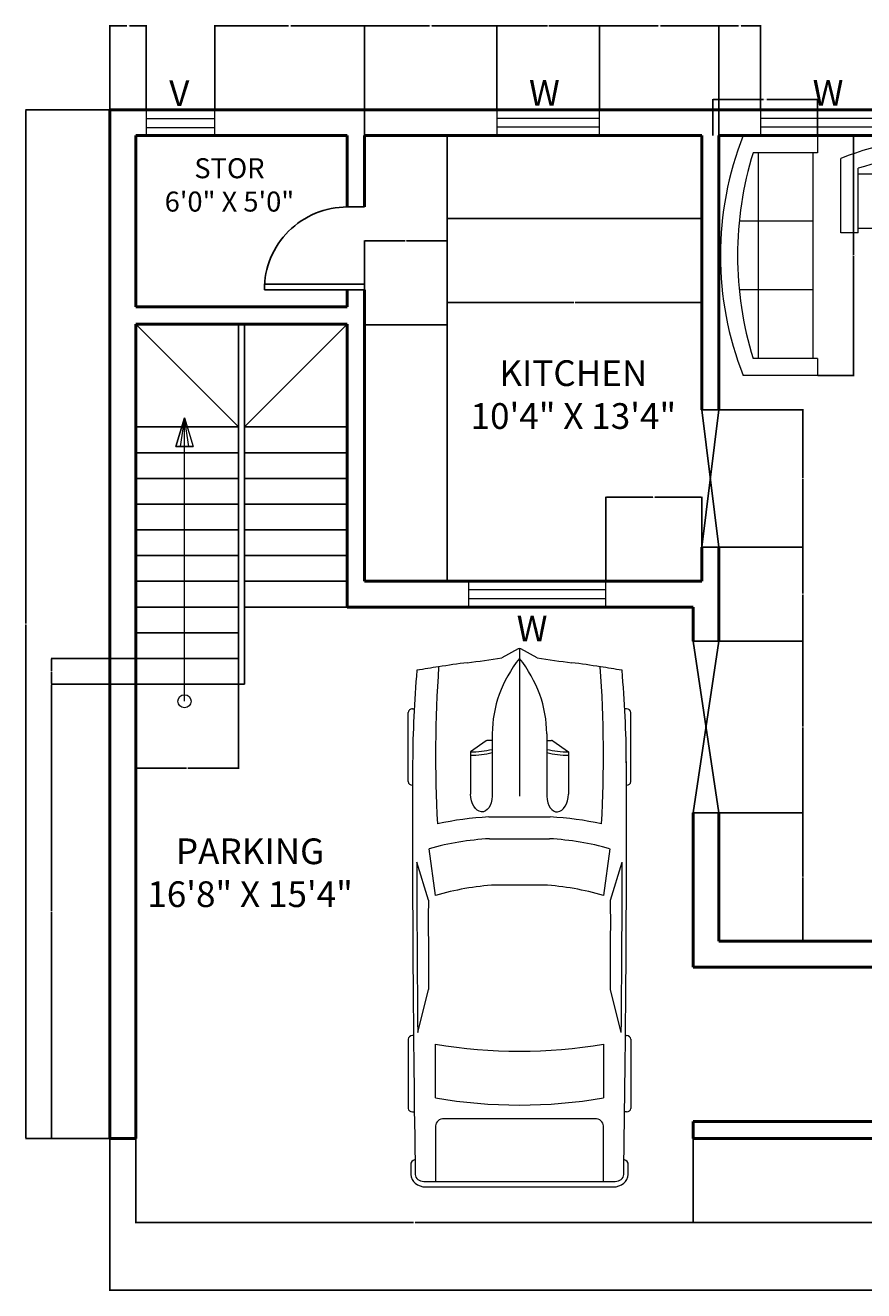
# Model space of a CAD drawing. Units: inches. Extents: x 1727 to 2326, y 1693 to 2164.
# Tile 1 of 3: x 1727 to 2020, y 1693 to 2136. Entities that reach past the tile are written whole.
import ezdxf

# ---------------------------------------------------------------- set-up
doc = ezdxf.new("R2010")
doc.units = ezdxf.units.IN
for name, color, linetype, lineweight in [('A-ANNO-DIMS', 2, 'Continuous', 18), ('A-ANNO-SYMB', 2, 'Continuous', 18), ('A-ANNO-TEXT', 3, 'Continuous', 18), ('A-AREA-IDEN', 7, 'Continuous', 25), ('A-DOOR', 3, 'Continuous', 25), ('A-EQPM-VEHI', 8, 'Continuous', 13), ('A-FLOR-CASE', 9, 'Continuous', 25), ('A-FLOR-STRS', 7, 'Continuous', 25), ('A-FURN', 8, 'Continuous', 18), ('A-GLAZ', 4, 'Continuous', 18), ('A-WALL', 7, 'Continuous', 50)]:
    doc.layers.add(name, color=color, linetype=linetype, lineweight=lineweight)
doc.styles.add('Annotative', font='arial.ttf')
doc.styles.get("Standard").update_dxf_attribs({"font": 'arial.ttf'})
doc.dimstyles.get("Standard").update_dxf_attribs({"dimtxt": 0.18, "dimasz": 0.18, "dimexe": 0.18, "dimexo": 0.0625, "dimgap": 0.09, "dimtad": 0, "dimtih": 1, "dimtoh": 1, "dimdec": 4, "dimzin": 0, "dimdsep": 46, "dimtxsty": 'Standard', "dimcen": 0.09, "dimadec": 0, "dimazin": 0, "dimtfac": 1, "dimtdec": 4, "dimtofl": 0, "dimtmove": 0, "dimatfit": 3, "dimfxl": 1, "dimtolj": 1, "dimtzin": 0, "dimarcsym": 0})

# ---------------------------------------------------------------- blocks, each defined once
blk = doc.blocks.new('Sofa - Roundback 7 ft.')
for p, q in [((-12.00002, -32.4421), (-12.00003, -6.5971)), ((11.99997, -32.4421), (11.99998, -6.5971)), ((-36.000027, -34), (-36.000027, -11.4696)), ((35.99998, -34), (35.99998, -11.4696)), ((-35.999844, -13.3819), (35.9998, -13.3819)), ((-36.000027, -32.4421), (35.99998, -32.4421))]:
    blk.add_line(p, q)
for points in [[(-36.000027, -34), (-42.000027, -34), (-42.000027, -8)], [(41.99998, -8), (41.99998, -34), (35.99998, -34)]]:
    blk.add_lwpolyline(points)
for centre, radius, start, end in [((0, -114.25), 114.25, 68.43141, 111.5686), ((-0.00001, -127.1968), 121.1968, 72.72033, 107.2797)]:
    blk.add_arc(centre, radius, start, end)
blk = doc.blocks.new('*U8')
for p, q in [((21.1, 37.41), (21.1, 36.83)), ((46.55, 38.89), (22.35, 38.89)), ((47.8, 37.39), (47.8, 37.41)), ((87.99, 31.87), (74.76, 35.92)), ((134.31, 35.6), (119.29, 31.78)), ((135.45, 37.07), (135.45, 37.41)), ((136.7, 38.89), (160.9, 38.89)), ((162.15, 37.41), (162.15, 36.77)), ((70.03, 31.54), (86.41, 29.35)), ((186.47, -33.5), (186.47, 33.5)), ((188.4, -32.76), (188.4, 32.76)), ((138.42, 29.35), (157.25, 29.35)), ((186.47, 29.35), (167.01, 29.35)), ((164.52, 26.39), (164.52, -26.39)), ((32.27, 11.63), (36.13, 17.17)), ((36.13, 17.17), (50.94, 17.17)), ((29.77, 9.51), (51.68, 9.51)), ((32.12, 9.51), (32.12, 11.15)), ((58.92, -10.77), (58.92, 10.77)), ((66.55, -10.53), (66.55, 10.53)), ((186.47, -10.53), (186.47, 10.53)), ((3.27, 6.13), (0.1, 0.41)), ((82.74, 8.5), (82.74, -8.5)), ((0, 0), (51.68, 0)), ((0.1, -0.41), (3.27, -6.13)), ((29.77, -9.51), (51.68, -9.51)), ((32.12, -9.51), (32.12, -11.15)), ((32.27, -11.63), (36.13, -17.17)), ((36.13, -17.17), (50.94, -17.17)), ((86.41, -29.35), (70.03, -31.54)), ((157.25, -29.35), (138.42, -29.35)), ((167.01, -29.35), (186.47, -29.35)), ((87.99, -31.87), (74.76, -35.92)), ((134.31, -35.6), (119.29, -31.78)), ((21.1, -37.41), (21.1, -36.83)), ((46.55, -38.89), (22.35, -38.89)), ((47.8, -37.39), (47.8, -37.41)), ((135.45, -37.07), (135.45, -37.41)), ((136.7, -38.89), (160.9, -38.89)), ((162.15, -37.41), (162.15, -36.77))]:
    blk.add_line(p, q)
for centre, major_axis, ratio, start_param, end_param in [((266.03, -27.52), (0, 313.31), 0.842304, 1.367076, 1.39176), ((41.19, -490.86), (0, 528.23), 0.842304, 0.00281, 0.075598), ((22.35, 37.41), (0, -1.48), 0.842304, 3.141593, 4.712389), ((64.48, -10555.62), (0, 10593.03), 0.842304, -0.013397, 0.002797), ((46.55, 37.41), (0, 1.48), 0.842304, -1.570796, 0), ((64.48, -10555.62), (0, -10591.55), 0.842304, 3.133765, 3.140441), ((136.7, 37.41), (0, -1.48), 0.842304, 3.141593, 4.712389), ((160.9, 37.41), (0, 1.48), 0.842304, -1.570796, 0), ((180.63, 35.84), (0, 2.22), 0.842304, -0.013017, 1.249894), ((64.48, -10556.36), (0, 10595.31), 0.842304, -0.013397, -0.013017), ((183.98, 33.5), (0, -2.96), 0.842304, 1.570796, 3.128196), ((183.98, 32.76), (0, -5.25), 0.842304, 1.570796, 3.128196), ((135.29, 5.39), (0, 81.77), 0.842304, 1.245306, 1.50788), ((95.79, -3666.35), (0, -3698.24), 0.842304, 3.134049, 3.144098), ((259.18, -27.52), (0, -305.3), 0.842304, 4.528606, 4.561838), ((37.47, -593.96), (0, -623.33), 0.842304, 3.096046, 3.200911), ((134.4, 5.39), (0, -89.78), 0.842304, 4.449482, 4.652344), ((149.6, 2.8), (0, -79.58), 0.842304, 4.372215, 4.640744), ((17.08, 0), (0, 147.02), 0.842304, 4.511394, 4.913384), ((35.91, 0), (0, 147.02), 0.842304, 4.511394, 4.913384), ((167.01, 26.39), (0, 2.96), 0.842304, 0, 1.570796), ((-204.49, 52.4), (0, -250.96), 0.842304, 1.385369, 1.434372), ((13.04, 17.01), (0, 27.42), 0.842304, 4.435146, 4.718221), ((14.2, 17.01), (0, 27.42), 0.842304, 4.435146, 4.718221), ((50.79, 13.34), (6.34, -0.36), 0.603834, -1.395552, 1.581315), ((29.77, -46.66), (0, 56.17), 0.842304, 0, 0.590319), ((32.75, 11.15), (0, 0.74), 0.842304, 0.879714, 1.570796), ((0.62, 0), (0, -0.74), 0.842304, 4.131459, 5.293319), ((29.77, 46.66), (0, 56.17), 0.842304, 2.551274, 3.141593), ((-204.49, -52.4), (0, 250.96), 0.842304, -1.434372, -1.385369), ((149.6, -2.8), (0, -79.58), 0.842304, -1.499151, -1.230623), ((32.75, -11.15), (0, -0.74), 0.842304, 4.712389, 5.403472), ((13.04, -17.01), (0, -27.42), 0.842304, 1.564964, 1.848039), ((14.2, -17.01), (0, -27.42), 0.842304, 1.564964, 1.848039), ((134.4, -5.39), (0, -89.78), 0.842304, -1.510751, -1.307889), ((135.29, -5.39), (0, -81.77), 0.842304, -1.50788, -1.245306), ((259.18, 27.52), (0, 305.3), 0.842304, 1.721348, 1.754579), ((167.01, -26.39), (0, -2.96), 0.842304, 4.712389, 6.283185), ((266.03, 27.52), (0, 313.31), 0.842304, 1.749832, 1.774517), ((37.47, 593.96), (0, -623.33), 0.842304, -0.059319, 0.045547), ((95.79, 3666.35), (0, -3698.24), 0.842304, -0.002505, 0.007544), ((183.98, -33.5), (0, 2.96), 0.842304, 3.15499, 4.712389), ((183.98, -32.76), (0, -5.25), 0.842304, 0.013397, 1.570796), ((41.19, 490.86), (0, -528.23), 0.842304, -0.075598, -0.00281), ((22.35, -37.41), (0, 1.48), 0.842304, 1.570796, 3.141593), ((64.48, 10555.62), (0, 10593.03), 0.842304, 3.138796, 3.15499), ((46.55, -37.41), (0, -1.48), 0.842304, 0, 1.570796), ((64.48, 10555.62), (0, -10591.55), 0.842304, 0.001152, 0.007828), ((136.7, -37.41), (0, -1.48), 0.842304, -1.570796, 0), ((160.9, -37.41), (0, 1.48), 0.842304, 3.141593, 4.712389), ((180.63, -35.84), (0, -2.22), 0.842304, -1.249894, 0.013017), ((64.48, 10556.36), (0, 10595.31), 0.842304, 3.15461, 3.15499)]:
    blk.add_ellipse(centre, major_axis=major_axis, ratio=ratio, start_param=start_param, end_param=end_param)
at = {"extrusion": (0, 0, -1)}
blk.add_ellipse((50.79, -13.34), major_axis=(6.34, 0.36), ratio=0.603834, start_param=-1.395552, end_param=1.581315, dxfattribs=at)
blk = doc.blocks.new('WIN-48IN')
for p, q in [((0, 48), (0, 0)), ((9, 48), (0, 48)), ((3, 48), (3, 0)), ((6, 0), (6, 48)), ((9, 0), (9, 48)), ((0, 0), (9, 0))]:
    blk.add_line(p, q)
blk = doc.blocks.new('DOOR-SWING-29IN')
for p, q in [((0, 29), (0, 35)), ((2, 29), (2, 35)), ((29, 35), (29, 29)), ((0, 29), (0, 0)), ((2, 29), (2, 0))]:
    blk.add_line(p, q)
blk.add_arc((0, 29), 29, 270, 0)
blk = doc.blocks.new('*D17')
at = {"layer": 'A-ANNO-DIMS', "color": 0, "lineweight": -2, "transparency": 16777216}
for p, q in [((2003.94, 2097.38), (2016.66, 2097.38)), ((2016.48, 2097.2), (2016.48, 2055.56)), ((2016.48, 2013.56), (2016.48, 2055.2)), ((2003.94, 2013.38), (2016.66, 2013.38))]:
    blk.add_line(p, q, dxfattribs=at)
at = {"layer": 'A-ANNO-DIMS', "color": 0, "transparency": 16777216}
for points in [[(2016.45, 2097.2), (2016.51, 2097.2), (2016.48, 2097.38)], [(2016.45, 2013.56), (2016.51, 2013.56), (2016.48, 2013.38)]]:
    blk.add_solid(points, dxfattribs=at)
at = {"layer": 'Defpoints', "color": 0, "transparency": 16777216}
for p in [(2003.88, 2097.38), (2016.48, 2097.38), (2003.88, 2013.38)]:
    blk.add_point(p, dxfattribs=at)
at = {"layer": 'A-ANNO-DIMS', "color": 0, "transparency": 16777216, "insert": (2016.48, 2055.38), "char_height": 0.18, "attachment_point": 5}
blk.add_mtext('\\A1;SOFA 84 TYP.', dxfattribs=at)
blk = doc.blocks.new('*D18')
at = {"layer": 'A-ANNO-DIMS', "color": 0, "lineweight": -2, "transparency": 16777216}
for p, q in [((1967.21, 2097.44), (1967.21, 2110.16)), ((1967.39, 2109.98), (1985.01, 2109.98)), ((2003.7, 2109.98), (1986.07, 2109.98)), ((2003.88, 2097.44), (2003.88, 2110.16))]:
    blk.add_line(p, q, dxfattribs=at)
at = {"layer": 'A-ANNO-DIMS', "color": 0, "transparency": 16777216}
for points in [[(1967.39, 2110.01), (1967.39, 2109.95), (1967.21, 2109.98)], [(2003.7, 2110.01), (2003.7, 2109.95), (2003.88, 2109.98)]]:
    blk.add_solid(points, dxfattribs=at)
at = {"layer": 'Defpoints', "color": 0, "transparency": 16777216}
for p in [(1967.21, 2109.98), (1967.21, 2097.38), (2003.88, 2097.38)]:
    blk.add_point(p, dxfattribs=at)
at = {"layer": 'A-ANNO-DIMS', "color": 0, "transparency": 16777216, "insert": (1985.54, 2109.98), "char_height": 0.18, "attachment_point": 5}
blk.add_mtext('\\A1;37 TYP.', dxfattribs=at)
blk = doc.blocks.new('*D33')
at = {"layer": 'A-ANNO-DIMS', "color": 0, "lineweight": -2, "transparency": 16777216}
for p, q in [((1756.37, 1746.32), (1756.37, 1693.11)), ((2296.37, 1746.32), (2296.37, 1693.11)), ((1756.55, 1693.29), (2026.08, 1693.29)), ((2296.19, 1693.29), (2026.66, 1693.29))]:
    blk.add_line(p, q, dxfattribs=at)
at = {"layer": 'A-ANNO-DIMS', "color": 0, "transparency": 16777216}
for points in [[(1756.55, 1693.32), (1756.55, 1693.26), (1756.37, 1693.29)], [(2296.19, 1693.32), (2296.19, 1693.26), (2296.37, 1693.29)]]:
    blk.add_solid(points, dxfattribs=at)
at = {"layer": 'Defpoints', "color": 0, "transparency": 16777216}
for p in [(1756.37, 1746.38), (2296.37, 1746.38), (2296.37, 1693.29)]:
    blk.add_point(p, dxfattribs=at)
at = {"layer": 'A-ANNO-DIMS', "color": 0, "transparency": 16777216, "insert": (2026.37, 1693.29), "char_height": 0.18, "attachment_point": 5}
blk.add_mtext('\\A1;540', dxfattribs=at)
blk = doc.blocks.new('*D34')
at = {"layer": 'A-ANNO-DIMS', "color": 0, "lineweight": -2, "transparency": 16777216}
for p, q in [((1756.31, 2106.38), (1726.79, 2106.38)), ((1726.97, 2106.2), (1726.97, 1926.56)), ((1726.97, 1746.56), (1726.97, 1926.2)), ((1756.31, 1746.38), (1726.79, 1746.38))]:
    blk.add_line(p, q, dxfattribs=at)
at = {"layer": 'A-ANNO-DIMS', "color": 0, "transparency": 16777216}
for points in [[(1726.94, 2106.2), (1727, 2106.2), (1726.97, 2106.38)], [(1726.94, 1746.56), (1727, 1746.56), (1726.97, 1746.38)]]:
    blk.add_solid(points, dxfattribs=at)
at = {"layer": 'Defpoints', "color": 0, "transparency": 16777216}
for p in [(1726.97, 2106.38), (1756.37, 2106.38), (1756.37, 1746.38)]:
    blk.add_point(p, dxfattribs=at)
at = {"layer": 'A-ANNO-DIMS', "color": 0, "transparency": 16777216, "insert": (1726.97, 1926.38), "char_height": 0.18, "attachment_point": 5}
blk.add_mtext('\\A1;360', dxfattribs=at)
blk = doc.blocks.new('*D35')
at = {"layer": 'A-ANNO-DIMS', "color": 0, "lineweight": -2, "transparency": 16777216}
for p, q in [((1756.37, 2106.44), (1756.37, 2135.96)), ((1756.55, 2135.78), (1762.26, 2135.78)), ((1768.88, 2135.78), (1763.17, 2135.78)), ((1769.06, 2106.25), (1769.06, 2135.96))]:
    blk.add_line(p, q, dxfattribs=at)
at = {"layer": 'A-ANNO-DIMS', "color": 0, "transparency": 16777216}
for points in [[(1756.55, 2135.81), (1756.55, 2135.75), (1756.37, 2135.78)], [(1768.88, 2135.81), (1768.88, 2135.75), (1769.06, 2135.78)]]:
    blk.add_solid(points, dxfattribs=at)
at = {"layer": 'Defpoints', "color": 0, "transparency": 16777216}
for p in [(1769.06, 2135.78), (1756.37, 2106.38), (1769.06, 2106.18)]:
    blk.add_point(p, dxfattribs=at)
at = {"layer": 'A-ANNO-DIMS', "color": 0, "transparency": 16777216, "insert": (1762.71, 2135.78), "char_height": 0.18, "attachment_point": 5}
blk.add_mtext('\\A1;12.683', dxfattribs=at)
blk = doc.blocks.new('*D36')
at = {"layer": 'A-ANNO-DIMS', "color": 0, "lineweight": -2, "transparency": 16777216}
for p, q in [((1793.06, 2106.25), (1793.06, 2135.96)), ((1793.24, 2135.78), (1818.82, 2135.78)), ((1845.19, 2135.78), (1819.61, 2135.78)), ((1845.37, 2097.44), (1845.37, 2135.96))]:
    blk.add_line(p, q, dxfattribs=at)
at = {"layer": 'A-ANNO-DIMS', "color": 0, "transparency": 16777216}
for points in [[(1793.24, 2135.81), (1793.24, 2135.75), (1793.06, 2135.78)], [(1845.19, 2135.81), (1845.19, 2135.75), (1845.37, 2135.78)]]:
    blk.add_solid(points, dxfattribs=at)
at = {"layer": 'Defpoints', "color": 0, "transparency": 16777216}
for p in [(1845.37, 2135.78), (1793.06, 2106.18), (1845.37, 2097.38)]:
    blk.add_point(p, dxfattribs=at)
at = {"layer": 'A-ANNO-DIMS', "color": 0, "transparency": 16777216, "insert": (1819.21, 2135.78), "char_height": 0.18, "attachment_point": 5}
blk.add_mtext('\\A1;52.32', dxfattribs=at)
blk = doc.blocks.new('*D37')
at = {"layer": 'A-ANNO-DIMS', "color": 0, "lineweight": -2, "transparency": 16777216}
for p, q in [((1845.37, 2097.44), (1845.37, 2135.96)), ((1845.55, 2135.78), (1868.11, 2135.78)), ((1891.45, 2135.78), (1868.9, 2135.78)), ((1891.63, 2106.44), (1891.63, 2135.96))]:
    blk.add_line(p, q, dxfattribs=at)
at = {"layer": 'A-ANNO-DIMS', "color": 0, "transparency": 16777216}
for points in [[(1845.55, 2135.81), (1845.55, 2135.75), (1845.37, 2135.78)], [(1891.45, 2135.81), (1891.45, 2135.75), (1891.63, 2135.78)]]:
    blk.add_solid(points, dxfattribs=at)
at = {"layer": 'Defpoints', "color": 0, "transparency": 16777216}
for p in [(1891.63, 2135.78), (1891.63, 2106.38), (1845.37, 2097.38)]:
    blk.add_point(p, dxfattribs=at)
at = {"layer": 'A-ANNO-DIMS', "color": 0, "transparency": 16777216, "insert": (1868.5, 2135.78), "char_height": 0.18, "attachment_point": 5}
blk.add_mtext('\\A1;46.26', dxfattribs=at)
blk = doc.blocks.new('*D38')
at = {"layer": 'A-ANNO-DIMS', "color": 0, "lineweight": -2, "transparency": 16777216}
for p, q in [((1891.63, 2106.44), (1891.63, 2135.96)), ((1891.81, 2135.78), (1909.42, 2135.78)), ((1927.45, 2135.78), (1909.85, 2135.78)), ((1927.63, 2106.44), (1927.63, 2135.96))]:
    blk.add_line(p, q, dxfattribs=at)
at = {"layer": 'A-ANNO-DIMS', "color": 0, "transparency": 16777216}
for points in [[(1891.81, 2135.81), (1891.81, 2135.75), (1891.63, 2135.78)], [(1927.45, 2135.81), (1927.45, 2135.75), (1927.63, 2135.78)]]:
    blk.add_solid(points, dxfattribs=at)
at = {"layer": 'Defpoints', "color": 0, "transparency": 16777216}
for p in [(1927.63, 2135.78), (1891.63, 2106.38), (1927.63, 2106.38)]:
    blk.add_point(p, dxfattribs=at)
at = {"layer": 'A-ANNO-DIMS', "color": 0, "transparency": 16777216, "insert": (1909.63, 2135.78), "char_height": 0.18, "attachment_point": 5}
blk.add_mtext('\\A1;36', dxfattribs=at)
blk = doc.blocks.new('*D39')
at = {"layer": 'A-ANNO-DIMS', "color": 0, "lineweight": -2, "transparency": 16777216}
for p, q in [((1927.63, 2106.44), (1927.63, 2135.96)), ((1927.81, 2135.78), (1948.11, 2135.78)), ((1969.19, 2135.78), (1948.9, 2135.78)), ((1969.37, 2097.44), (1969.37, 2135.96))]:
    blk.add_line(p, q, dxfattribs=at)
at = {"layer": 'A-ANNO-DIMS', "color": 0, "transparency": 16777216}
for points in [[(1927.81, 2135.81), (1927.81, 2135.75), (1927.63, 2135.78)], [(1969.19, 2135.81), (1969.19, 2135.75), (1969.37, 2135.78)]]:
    blk.add_solid(points, dxfattribs=at)
at = {"layer": 'Defpoints', "color": 0, "transparency": 16777216}
for p in [(1969.37, 2135.78), (1927.63, 2106.38), (1969.37, 2097.38)]:
    blk.add_point(p, dxfattribs=at)
at = {"layer": 'A-ANNO-DIMS', "color": 0, "transparency": 16777216, "insert": (1948.5, 2135.78), "char_height": 0.18, "attachment_point": 5}
blk.add_mtext('\\A1;41.74', dxfattribs=at)
blk = doc.blocks.new('*D40')
at = {"layer": 'A-ANNO-DIMS', "color": 0, "lineweight": -2, "transparency": 16777216}
for p, q in [((1969.37, 2097.44), (1969.37, 2135.96)), ((1969.55, 2135.78), (1976.2, 2135.78)), ((1983.76, 2135.78), (1977.11, 2135.78)), ((1983.94, 2106.44), (1983.94, 2135.96))]:
    blk.add_line(p, q, dxfattribs=at)
at = {"layer": 'A-ANNO-DIMS', "color": 0, "transparency": 16777216}
for points in [[(1969.55, 2135.81), (1969.55, 2135.75), (1969.37, 2135.78)], [(1983.76, 2135.81), (1983.76, 2135.75), (1983.94, 2135.78)]]:
    blk.add_solid(points, dxfattribs=at)
at = {"layer": 'Defpoints', "color": 0, "transparency": 16777216}
for p in [(1983.94, 2135.78), (1983.94, 2106.38), (1969.37, 2097.38)]:
    blk.add_point(p, dxfattribs=at)
at = {"layer": 'A-ANNO-DIMS', "color": 0, "transparency": 16777216, "insert": (1976.65, 2135.78), "char_height": 0.18, "attachment_point": 5}
blk.add_mtext('\\A1;14.563', dxfattribs=at)
blk = doc.blocks.new('*D51')
at = {"layer": 'A-ANNO-DIMS', "color": 0, "lineweight": -2, "transparency": 16777216}
for p, q in [((1765.37, 1905.32), (1765.37, 1875.8)), ((1801.37, 1905.32), (1801.37, 1875.8)), ((1765.55, 1875.98), (1783.15, 1875.98)), ((1801.19, 1875.98), (1783.59, 1875.98))]:
    blk.add_line(p, q, dxfattribs=at)
at = {"layer": 'A-ANNO-DIMS', "color": 0, "transparency": 16777216}
for points in [[(1765.55, 1876.01), (1765.55, 1875.95), (1765.37, 1875.98)], [(1801.19, 1876.01), (1801.19, 1875.95), (1801.37, 1875.98)]]:
    blk.add_solid(points, dxfattribs=at)
at = {"layer": 'Defpoints', "color": 0, "transparency": 16777216}
for p in [(1765.37, 1905.38), (1801.37, 1905.38), (1765.37, 1875.98)]:
    blk.add_point(p, dxfattribs=at)
at = {"layer": 'A-ANNO-DIMS', "color": 0, "transparency": 16777216, "insert": (1783.37, 1875.98), "char_height": 0.18, "attachment_point": 5}
blk.add_mtext('\\A1;36', dxfattribs=at)
blk = doc.blocks.new('*D52')
at = {"layer": 'A-ANNO-DIMS', "color": 0, "lineweight": -2, "transparency": 16777216}
for p, q in [((1765.31, 1914.38), (1735.79, 1914.38)), ((1735.97, 1914.2), (1735.97, 1910.06)), ((1735.97, 1905.56), (1735.97, 1909.7)), ((1765.31, 1905.38), (1735.79, 1905.38))]:
    blk.add_line(p, q, dxfattribs=at)
at = {"layer": 'A-ANNO-DIMS', "color": 0, "transparency": 16777216}
for points in [[(1735.94, 1914.2), (1736, 1914.2), (1735.97, 1914.38)], [(1735.94, 1905.56), (1736, 1905.56), (1735.97, 1905.38)]]:
    blk.add_solid(points, dxfattribs=at)
at = {"layer": 'Defpoints', "color": 0, "transparency": 16777216}
for p in [(1735.97, 1914.38), (1765.37, 1914.38), (1765.37, 1905.38)]:
    blk.add_point(p, dxfattribs=at)
at = {"layer": 'A-ANNO-DIMS', "color": 0, "transparency": 16777216, "insert": (1735.97, 1909.88), "char_height": 0.18, "attachment_point": 5}
blk.add_mtext('\\A1;9', dxfattribs=at)
blk = doc.blocks.new('*D53')
at = {"layer": 'A-ANNO-DIMS', "color": 0, "lineweight": -2, "transparency": 16777216}
for p, q in [((1765.31, 1905.38), (1735.79, 1905.38)), ((1735.97, 1905.2), (1735.97, 1826.06)), ((1735.97, 1746.56), (1735.97, 1825.7)), ((1765.31, 1746.38), (1735.79, 1746.38))]:
    blk.add_line(p, q, dxfattribs=at)
at = {"layer": 'A-ANNO-DIMS', "color": 0, "transparency": 16777216}
for points in [[(1735.94, 1905.2), (1736, 1905.2), (1735.97, 1905.38)], [(1735.94, 1746.56), (1736, 1746.56), (1735.97, 1746.38)]]:
    blk.add_solid(points, dxfattribs=at)
at = {"layer": 'Defpoints', "color": 0, "transparency": 16777216}
for p in [(1735.97, 1905.38), (1765.37, 1905.38), (1765.37, 1746.38)]:
    blk.add_point(p, dxfattribs=at)
at = {"layer": 'A-ANNO-DIMS', "color": 0, "transparency": 16777216, "insert": (1735.97, 1825.88), "char_height": 0.18, "attachment_point": 5}
blk.add_mtext('\\A1;159', dxfattribs=at)
blk = doc.blocks.new('*D55')
at = {"layer": 'A-ANNO-DIMS', "color": 0, "lineweight": -2, "transparency": 16777216}
for p, q in [((1765.37, 1746.32), (1765.37, 1716.8)), ((1960.37, 1746.32), (1960.37, 1716.8)), ((1765.55, 1716.98), (1862.59, 1716.98)), ((1960.19, 1716.98), (1863.15, 1716.98))]:
    blk.add_line(p, q, dxfattribs=at)
at = {"layer": 'A-ANNO-DIMS', "color": 0, "transparency": 16777216}
for points in [[(1765.55, 1717.01), (1765.55, 1716.95), (1765.37, 1716.98)], [(1960.19, 1717.01), (1960.19, 1716.95), (1960.37, 1716.98)]]:
    blk.add_solid(points, dxfattribs=at)
at = {"layer": 'Defpoints', "color": 0, "transparency": 16777216}
for p in [(1765.37, 1746.38), (1960.37, 1746.38), (1765.37, 1716.98)]:
    blk.add_point(p, dxfattribs=at)
at = {"layer": 'A-ANNO-DIMS', "color": 0, "transparency": 16777216, "insert": (1862.87, 1716.98), "char_height": 0.18, "attachment_point": 5}
blk.add_mtext('\\A1;195', dxfattribs=at)
blk = doc.blocks.new('*D56')
at = {"layer": 'A-ANNO-DIMS', "color": 0, "lineweight": -2, "transparency": 16777216}
for p, q in [((1960.37, 1746.32), (1960.37, 1716.8)), ((2134.37, 1746.32), (2134.37, 1716.8)), ((1960.55, 1716.98), (2047.09, 1716.98)), ((2134.19, 1716.98), (2047.65, 1716.98))]:
    blk.add_line(p, q, dxfattribs=at)
at = {"layer": 'A-ANNO-DIMS', "color": 0, "transparency": 16777216}
for points in [[(1960.55, 1717.01), (1960.55, 1716.95), (1960.37, 1716.98)], [(2134.19, 1717.01), (2134.19, 1716.95), (2134.37, 1716.98)]]:
    blk.add_solid(points, dxfattribs=at)
at = {"layer": 'Defpoints', "color": 0, "transparency": 16777216}
for p in [(1960.37, 1746.38), (2134.37, 1746.38), (1960.37, 1716.98)]:
    blk.add_point(p, dxfattribs=at)
at = {"layer": 'A-ANNO-DIMS', "color": 0, "transparency": 16777216, "insert": (2047.37, 1716.98), "char_height": 0.18, "attachment_point": 5}
blk.add_mtext('\\A1;174', dxfattribs=at)
blk = doc.blocks.new('*D59')
at = {"layer": 'A-ANNO-DIMS', "color": 0, "lineweight": -2, "transparency": 16777216}
for p, q in [((1969.44, 2001.38), (1998.95, 2001.38)), ((1998.77, 2001.2), (1998.77, 1977.56)), ((1998.77, 1953.56), (1998.77, 1977.2)), ((1969.44, 1953.38), (1998.95, 1953.38))]:
    blk.add_line(p, q, dxfattribs=at)
at = {"layer": 'A-ANNO-DIMS', "color": 0, "transparency": 16777216}
for points in [[(1998.74, 2001.2), (1998.8, 2001.2), (1998.77, 2001.38)], [(1998.74, 1953.56), (1998.8, 1953.56), (1998.77, 1953.38)]]:
    blk.add_solid(points, dxfattribs=at)
at = {"layer": 'Defpoints', "color": 0, "transparency": 16777216}
for p in [(1969.37, 2001.38), (1969.37, 1953.38), (1998.77, 1953.38)]:
    blk.add_point(p, dxfattribs=at)
at = {"layer": 'A-ANNO-DIMS', "color": 0, "transparency": 16777216, "insert": (1998.77, 1977.38), "char_height": 0.18, "attachment_point": 5}
blk.add_mtext('\\A1;48', dxfattribs=at)
blk = doc.blocks.new('*D60')
at = {"layer": 'A-ANNO-DIMS', "color": 0, "lineweight": -2, "transparency": 16777216}
for p, q in [((1969.44, 1953.38), (1998.95, 1953.38)), ((1998.77, 1953.2), (1998.77, 1937.06)), ((1998.77, 1920.56), (1998.77, 1936.7)), ((1969.44, 1920.38), (1998.95, 1920.38))]:
    blk.add_line(p, q, dxfattribs=at)
at = {"layer": 'A-ANNO-DIMS', "color": 0, "transparency": 16777216}
for points in [[(1998.74, 1953.2), (1998.8, 1953.2), (1998.77, 1953.38)], [(1998.74, 1920.56), (1998.8, 1920.56), (1998.77, 1920.38)]]:
    blk.add_solid(points, dxfattribs=at)
at = {"layer": 'Defpoints', "color": 0, "transparency": 16777216}
for p in [(1969.37, 1953.38), (1969.37, 1920.38), (1998.77, 1920.38)]:
    blk.add_point(p, dxfattribs=at)
at = {"layer": 'A-ANNO-DIMS', "color": 0, "transparency": 16777216, "insert": (1998.77, 1936.88), "char_height": 0.18, "attachment_point": 5}
blk.add_mtext('\\A1;33', dxfattribs=at)
blk = doc.blocks.new('*D61')
at = {"layer": 'A-ANNO-DIMS', "color": 0, "lineweight": -2, "transparency": 16777216}
for p, q in [((1969.44, 1920.38), (1998.95, 1920.38)), ((1998.77, 1920.2), (1998.77, 1890.56)), ((1998.77, 1860.56), (1998.77, 1890.2)), ((1969.44, 1860.38), (1998.95, 1860.38))]:
    blk.add_line(p, q, dxfattribs=at)
at = {"layer": 'A-ANNO-DIMS', "color": 0, "transparency": 16777216}
for points in [[(1998.74, 1920.2), (1998.8, 1920.2), (1998.77, 1920.38)], [(1998.74, 1860.56), (1998.8, 1860.56), (1998.77, 1860.38)]]:
    blk.add_solid(points, dxfattribs=at)
at = {"layer": 'Defpoints', "color": 0, "transparency": 16777216}
for p in [(1969.37, 1920.38), (1969.37, 1860.38), (1998.77, 1860.38)]:
    blk.add_point(p, dxfattribs=at)
at = {"layer": 'A-ANNO-DIMS', "color": 0, "transparency": 16777216, "insert": (1998.77, 1890.38), "char_height": 0.18, "attachment_point": 5}
blk.add_mtext('\\A1;60', dxfattribs=at)
blk = doc.blocks.new('*D62')
at = {"layer": 'A-ANNO-DIMS', "color": 0, "lineweight": -2, "transparency": 16777216}
for p, q in [((1969.44, 1860.38), (1998.95, 1860.38)), ((1998.77, 1860.2), (1998.77, 1838.06)), ((1998.77, 1815.56), (1998.77, 1837.7)), ((1969.44, 1815.38), (1998.95, 1815.38))]:
    blk.add_line(p, q, dxfattribs=at)
at = {"layer": 'A-ANNO-DIMS', "color": 0, "transparency": 16777216}
for points in [[(1998.74, 1860.2), (1998.8, 1860.2), (1998.77, 1860.38)], [(1998.74, 1815.56), (1998.8, 1815.56), (1998.77, 1815.38)]]:
    blk.add_solid(points, dxfattribs=at)
at = {"layer": 'Defpoints', "color": 0, "transparency": 16777216}
for p in [(1969.37, 1860.38), (1969.37, 1815.38), (1998.77, 1815.38)]:
    blk.add_point(p, dxfattribs=at)
at = {"layer": 'A-ANNO-DIMS', "color": 0, "transparency": 16777216, "insert": (1998.77, 1837.88), "char_height": 0.18, "attachment_point": 5}
blk.add_mtext('\\A1;45', dxfattribs=at)
blk = doc.blocks.new('*D64')
at = {"layer": 'A-ANNO-DIMS', "color": 0, "lineweight": -2, "transparency": 16777216}
for p, q in [((1929.81, 1941.44), (1929.81, 1970.96)), ((1929.99, 1970.78), (1946.2, 1970.78)), ((1963.19, 1970.78), (1946.99, 1970.78)), ((1963.37, 1941.44), (1963.37, 1970.96))]:
    blk.add_line(p, q, dxfattribs=at)
at = {"layer": 'A-ANNO-DIMS', "color": 0, "transparency": 16777216}
for points in [[(1929.99, 1970.81), (1929.99, 1970.75), (1929.81, 1970.78)], [(1963.19, 1970.81), (1963.19, 1970.75), (1963.37, 1970.78)]]:
    blk.add_solid(points, dxfattribs=at)
at = {"layer": 'Defpoints', "color": 0, "transparency": 16777216}
for p in [(1963.37, 1970.78), (1929.81, 1941.38), (1963.37, 1941.38)]:
    blk.add_point(p, dxfattribs=at)
at = {"layer": 'A-ANNO-DIMS', "color": 0, "transparency": 16777216, "insert": (1946.59, 1970.78), "char_height": 0.18, "attachment_point": 5}
blk.add_mtext('\\A1;33.56', dxfattribs=at)
blk = doc.blocks.new('*D65')
at = {"layer": 'A-ANNO-DIMS', "color": 0, "lineweight": -2, "transparency": 16777216}
for p, q in [((1874.37, 2068.32), (1874.37, 2038.8)), ((1963.37, 2068.32), (1963.37, 2038.8)), ((1874.55, 2038.98), (1918.65, 2038.98)), ((1963.19, 2038.98), (1919.09, 2038.98))]:
    blk.add_line(p, q, dxfattribs=at)
at = {"layer": 'A-ANNO-DIMS', "color": 0, "transparency": 16777216}
for points in [[(1874.55, 2039.01), (1874.55, 2038.95), (1874.37, 2038.98)], [(1963.19, 2039.01), (1963.19, 2038.95), (1963.37, 2038.98)]]:
    blk.add_solid(points, dxfattribs=at)
at = {"layer": 'Defpoints', "color": 0, "transparency": 16777216}
for p in [(1874.37, 2068.38), (1963.37, 2068.38), (1874.37, 2038.98)]:
    blk.add_point(p, dxfattribs=at)
at = {"layer": 'A-ANNO-DIMS', "color": 0, "transparency": 16777216, "insert": (1918.87, 2038.98), "char_height": 0.18, "attachment_point": 5}
blk.add_mtext('\\A1;89', dxfattribs=at)
blk = doc.blocks.new('*D66')
at = {"layer": 'A-ANNO-DIMS', "color": 0, "lineweight": -2, "transparency": 16777216}
for p, q in [((1845.37, 2031.16), (1845.37, 2060.68)), ((1845.55, 2060.5), (1859.65, 2060.5)), ((1874.19, 2060.5), (1860.09, 2060.5)), ((1874.37, 2031.16), (1874.37, 2060.68))]:
    blk.add_line(p, q, dxfattribs=at)
at = {"layer": 'A-ANNO-DIMS', "color": 0, "transparency": 16777216}
for points in [[(1845.55, 2060.53), (1845.55, 2060.47), (1845.37, 2060.5)], [(1874.19, 2060.53), (1874.19, 2060.47), (1874.37, 2060.5)]]:
    blk.add_solid(points, dxfattribs=at)
at = {"layer": 'Defpoints', "color": 0, "transparency": 16777216}
for p in [(1874.37, 2060.5), (1845.37, 2031.1), (1874.37, 2031.1)]:
    blk.add_point(p, dxfattribs=at)
at = {"layer": 'A-ANNO-DIMS', "color": 0, "transparency": 16777216, "insert": (1859.87, 2060.5), "char_height": 0.18, "attachment_point": 5}
blk.add_mtext('\\A1;29', dxfattribs=at)

msp = doc.modelspace()

# ---------------------------------------------------------------- linework, layer by layer
at = {"layer": 'A-ANNO-SYMB'}
for p, q in [((1782.4415, 1998.5763), (1779.4415, 1988.5763)), ((1779.4415, 1988.5763), (1782.4415, 1998.5763)), ((1782.4415, 1998.5763), (1780.9415, 1988.5763)), ((1782.4415, 1988.5763), (1782.4415, 1998.5763)), ((1782.4415, 1998.5763), (1785.4415, 1988.5763)), ((1783.9415, 1988.5763), (1782.4415, 1998.5763)), ((1782.4415, 1988.5763), (1779.4415, 1988.5763)), ((1779.4415, 1988.5763), (1782.4415, 1988.5763)), ((1782.4415, 1899.3942), (1782.4415, 1988.5763)), ((1782.4415, 1988.5763), (1785.4415, 1988.5763)), ((1785.4415, 1988.5763), (1782.4415, 1988.5763)), ((1785.4415, 1988.5763), (1783.9415, 1988.5763))]:
    msp.add_line(p, q, dxfattribs=at)
msp.add_circle((1782.4415, 1899.3942), 2.2869, dxfattribs=at)
at = {"layer": 'A-DOOR'}
for p, q in [((1969.3729, 2001.3813), (1963.3729, 2001.3813)), ((1963.3729, 1953.3813), (1969.3729, 2001.3813)), ((1969.3729, 2001.3813), (1963.3729, 2001.3813)), ((1963.3729, 2001.3813), (1969.3729, 1953.3813)), ((1963.3729, 1953.3813), (1969.3729, 1953.3813)), ((1960.3729, 1920.3813), (1969.3729, 1920.3813)), ((1960.3729, 1860.3813), (1969.3729, 1920.3813)), ((1969.3729, 1920.3813), (1960.3729, 1920.3813)), ((1960.3729, 1920.3813), (1969.3729, 1860.3813)), ((1969.3729, 1860.3813), (1960.3729, 1860.3813))]:
    msp.add_line(p, q, dxfattribs=at)
at = {"layer": 'A-FLOR-CASE'}
for p, q in [((1874.3729, 2097.3813), (1874.3729, 2068.3813)), ((1874.3729, 2068.3813), (1963.3729, 2068.3813)), ((1845.3729, 2031.101), (1874.3729, 2031.101)), ((1874.3729, 2031.101), (1874.3729, 1941.3813))]:
    msp.add_line(p, q, dxfattribs=at)
at = {"layer": 'A-FLOR-STRS'}
for p, q in [((1801.3729, 1995.3813), (1765.3729, 2031.3813)), ((1765.3729, 2031.3813), (1786.3741, 2031.3813)), ((1801.3729, 1905.3813), (1801.3729, 2031.3813)), ((1803.3729, 1905.3813), (1803.3729, 2031.3813)), ((1803.3729, 1995.3813), (1839.3729, 2031.3813)), ((1765.3729, 1995.3813), (1801.3729, 1995.3813)), ((1803.3729, 1995.3813), (1839.3729, 1995.3813)), ((1765.3729, 1986.3813), (1801.3729, 1986.3813)), ((1803.3729, 1986.3813), (1839.3729, 1986.3813)), ((1765.3729, 1977.3813), (1801.3729, 1977.3813)), ((1803.3729, 1977.3813), (1839.3729, 1977.3813)), ((1765.3729, 1968.3813), (1801.3729, 1968.3813)), ((1803.3729, 1968.3813), (1839.3729, 1968.3813)), ((1765.3729, 1959.3813), (1801.3729, 1959.3813)), ((1803.3729, 1959.3813), (1839.3729, 1959.3813)), ((1765.3729, 1950.3813), (1801.3729, 1950.3813)), ((1803.3729, 1950.3813), (1839.3729, 1950.3813)), ((1765.3729, 1941.3813), (1801.3729, 1941.3813)), ((1803.3729, 1941.3813), (1839.3729, 1941.3813)), ((1765.3729, 1932.3813), (1801.3729, 1932.3813)), ((1803.3729, 1932.3813), (1839.3729, 1932.3813)), ((1765.3729, 1923.3813), (1801.3729, 1923.3813)), ((1765.3729, 1914.3813), (1801.3729, 1914.3813)), ((1765.3729, 1905.3813), (1803.3729, 1905.3813))]:
    msp.add_line(p, q, dxfattribs=at)
at = {"layer": 'A-GLAZ'}
for p, q in [((1769.0559, 2106.1833), (1769.0559, 2097.1833)), ((1793.0559, 2097.1833), (1793.0559, 2106.1833)), ((1927.6343, 2106.3813), (1879.6343, 2106.3813)), ((1891.6343, 2106.3813), (1891.6343, 2097.3813)), ((1927.6343, 2097.3813), (1927.6343, 2106.3813)), ((1793.0559, 2103.1833), (1769.0559, 2103.1833)), ((1769.0559, 2100.1833), (1793.0559, 2100.1833)), ((1927.6343, 2103.3813), (1891.6343, 2103.3813)), ((1891.6343, 2100.3813), (1927.6343, 2100.3813)), ((1879.6343, 2097.3813), (1927.6343, 2097.3813))]:
    msp.add_line(p, q, dxfattribs=at)
at = {"layer": 'A-WALL'}
for p, q in [((1756.3729, 2106.3813), (2296.3729, 2106.3813)), ((1756.3729, 1746.3813), (1756.3729, 2106.3813)), ((1756.3729, 2106.3813), (1765.3729, 2106.3813)), ((1765.3729, 2097.3813), (1839.3729, 2097.3813)), ((1765.3729, 2037.3813), (1765.3729, 2097.3813)), ((1839.3729, 2097.3813), (1839.3729, 2072.3813)), ((1845.3729, 2097.3813), (1845.3729, 2072.3813)), ((1845.3729, 2097.3813), (1963.3729, 2097.3813)), ((1963.3729, 2097.3813), (1963.3729, 2001.3813)), ((1969.3729, 2097.3813), (1969.3729, 2001.3813)), ((1969.3729, 2097.3813), (2137.3729, 2097.3813)), ((1839.3729, 2037.3813), (1839.3729, 2043.3813)), ((1839.3729, 2043.3813), (1839.3729, 2037.3813)), ((1845.3729, 2043.3813), (1845.3729, 1941.3813)), ((1765.3729, 2037.3813), (1839.3729, 2037.3813)), ((1765.3729, 1755.3813), (1765.3729, 2031.3813)), ((1765.3729, 2031.3813), (1839.3729, 2031.3813)), ((1839.3729, 2031.3813), (1839.3729, 1941.3813)), ((1963.3729, 1941.3813), (1963.3729, 1953.3813)), ((1963.3729, 1953.3813), (1963.3729, 1941.3813)), ((1969.3729, 1953.3813), (1969.3729, 1941.3813)), ((1839.3729, 1941.3813), (1839.3729, 1932.3813)), ((1845.3729, 1941.3813), (1963.3729, 1941.3813)), ((1969.3729, 1941.3813), (1969.3729, 1927.4801)), ((1839.3729, 1932.3813), (1960.3729, 1932.3813)), ((1960.3729, 1932.3813), (1960.3729, 1920.3813)), ((1960.3729, 1932.3813), (1960.3729, 1920.3813)), ((1969.3729, 1932.3813), (1969.3729, 1920.3813)), ((1960.3729, 1860.3813), (1960.3729, 1806.3813)), ((1969.3729, 1860.3813), (1969.3729, 1815.3813)), ((1969.3729, 1815.3813), (2047.3729, 1815.3813)), ((1963.3729, 1806.3813), (1960.3729, 1806.3813)), ((1963.3729, 1806.3813), (2134.3729, 1806.3813)), ((1765.3729, 1755.3813), (1765.3729, 1746.3813)), ((1960.3729, 1752.3813), (1960.3729, 1746.3813)), ((2134.3729, 1752.3813), (1960.3729, 1752.3813)), ((1765.3729, 1746.3813), (1756.3729, 1746.3813)), ((2296.3729, 1746.3813), (1960.3729, 1746.3813))]:
    msp.add_line(p, q, dxfattribs=at)

# ---------------------------------------------------------------- block references
at = {"layer": 'A-DOOR', "extrusion": (0, 0, -1), "zscale": -1, "rotation": 89.99999999999937}
msp.add_blockref('DOOR-SWING-29IN', (-1810.3726, 2043.3814), dxfattribs=at)
at = {"layer": 'A-EQPM-VEHI', "rotation": 270}
msp.add_blockref('*U8', (1899.6143, 1917.8239), dxfattribs=at)
at = {"layer": 'A-FURN'}
msp.add_blockref('Sofa - Roundback 7 ft.', (2054.0432, 2097.3813), dxfattribs=at)
at = {"layer": 'A-FURN', "rotation": 90}
msp.add_blockref('Sofa - Roundback 7 ft.', (1969.8756, 2055.3814), dxfattribs=at)
at = {"layer": 'A-GLAZ'}
for p, rotation in [((1983.936, 2106.3812), 270.0000000000012), ((1881.8142, 1941.3812), 269.9999999999983)]:
    msp.add_blockref('WIN-48IN', p, dxfattribs=dict(at, rotation=rotation))

# ---------------------------------------------------------------- texts
at = {"layer": 'A-ANNO-TEXT', "char_height": 9, "width": 33.967268, "attachment_point": 1, "style": 'Annotative'}
for s, insert in [('\\pxqc;V', (1763.6348, 2116.7193)), ('\\pxqc;W', (1891.3398, 2116.795)), ('\\pxqc;W', (1990.5516, 2116.8101)), ('\\pxqc;W', (1887.0324, 1929.3298))]:
    msp.add_mtext(s, dxfattribs=dict(at, insert=insert))
at = {"layer": 'A-AREA-IDEN', "attachment_point": 1, "style": 'Annotative'}
for s, insert, char_height, width in [('\\pxqc;STOR\\P6\'0" X 5\'0"', (1769.8242, 2089.4393), 7, 56.677462), ('\\pxqc;KITCHEN\\P10\'4" X 13\'4"', (1853.4478, 2018.7259), 9, 130.001559), ('\\pxqc;PARKING\\P16\'8" X 15\'4"', (1740.378, 1851.3851), 9, 130.001559)]:
    msp.add_mtext(s, dxfattribs=dict(at, insert=insert, char_height=char_height, width=width))

# ---------------------------------------------------------------- dimensions: what is measured, and where the dimension line sits
at = {"layer": 'A-ANNO-DIMS'}
for base, p1, p2, override, picture, middle in [((1769.0559, 2135.7813), (1756.3729, 2106.3813), (1769.0559, 2106.1833), {"dimdec": 3, "dimlfac": 1, "dimrnd": 0, "dimzin": 0, "dimdsep": 46, "dimlunit": 2}, '*D35', (1762.7144, 2135.7813)), ((1845.3729, 2135.7813), (1793.0559, 2106.1833), (1845.3729, 2097.3813), {"dimdec": 2, "dimlfac": 1, "dimrnd": 0, "dimzin": 0, "dimdsep": 46, "dimlunit": 2}, '*D36', (1819.2144, 2135.7813)), ((1891.6343, 2135.7813), (1845.3729, 2097.3813), (1891.6343, 2106.3813), {"dimdec": 2, "dimlfac": 1, "dimrnd": 0, "dimzin": 0, "dimdsep": 46, "dimlunit": 2}, '*D37', (1868.5036, 2135.7813)), ((1927.6343, 2135.7813), (1891.6343, 2106.3813), (1927.6343, 2106.3813), {"dimdec": 0, "dimlfac": 1, "dimrnd": 0, "dimzin": 0, "dimdsep": 46, "dimlunit": 2}, '*D38', (1909.6343, 2135.7813)), ((1969.3729, 2135.7813), (1927.6343, 2106.3813), (1969.3729, 2097.3813), {"dimdec": 2, "dimlfac": 1, "dimrnd": 0, "dimzin": 0, "dimdsep": 46, "dimlunit": 2}, '*D39', (1948.5036, 2135.7813)), ((1983.9357, 2135.7813), (1969.3729, 2097.3813), (1983.9357, 2106.3813), {"dimdec": 3, "dimlfac": 1, "dimrnd": 0, "dimzin": 0, "dimdsep": 46, "dimlunit": 2}, '*D40', (1976.6543, 2135.7813)), ((1874.3729, 2060.501), (1845.3729, 2031.101), (1874.3729, 2031.101), {"dimdec": 0, "dimlfac": 1, "dimrnd": 0, "dimzin": 0, "dimdsep": 46, "dimlunit": 2}, '*D66', (1859.8729, 2060.501)), ((1963.3729, 1970.7813), (1929.8139, 1941.3813), (1963.3729, 1941.3813), {"dimdec": 2, "dimlfac": 1, "dimrnd": 0, "dimzin": 0, "dimdsep": 46, "dimlunit": 2}, '*D64', (1946.5934, 1970.7813)), ((2296.3729, 1693.2922), (1756.3729, 1746.3813), (2296.3729, 1746.3813), {"dimdec": 0, "dimlfac": 1, "dimrnd": 0, "dimzin": 0, "dimdsep": 46, "dimlunit": 2}, '*D33', (2026.3729, 1693.2922))]:
    dim = msp.add_linear_dim(base=base, p1=p1, p2=p2, dimstyle='Standard', override=override, dxfattribs=at)
    dim.commit()
    dim.dimension.update_dxf_attribs({"geometry": picture, "text_midpoint": middle})
for base, p1, p2, angle, text, picture, middle in [((1967.209, 2109.9813), (2003.8756, 2097.3813), (1967.209, 2097.3813), 180, '<> TYP.', '*D18', (1985.5423, 2109.9813)), ((2016.4756, 2097.3813), (2003.8756, 2013.3813), (2003.8756, 2097.3813), 90, 'SOFA <> TYP.', '*D17', (2016.4756, 2055.3813))]:
    dim = msp.add_linear_dim(base=base, p1=p1, p2=p2, angle=angle, text=text, dimstyle='Standard', override={"dimdec": 0, "dimlfac": 1, "dimrnd": 0, "dimzin": 0, "dimdsep": 46, "dimlunit": 2}, dxfattribs=at)
    dim.commit()
    dim.dimension.update_dxf_attribs({"geometry": picture, "text_midpoint": middle})
for base, p1, p2, angle, picture, middle in [((1726.9729, 2106.3813), (1756.3729, 1746.3813), (1756.3729, 2106.3813), 90, '*D34', (1726.9729, 1926.3813)), ((1874.3729, 2038.9813), (1963.3729, 2068.3813), (1874.3729, 2068.3813), 180, '*D65', (1918.8729, 2038.9813)), ((1998.7729, 1953.3813), (1969.3729, 2001.3813), (1969.3729, 1953.3813), 270, '*D59', (1998.7729, 1977.3813)), ((1998.7729, 1920.3813), (1969.3729, 1953.3813), (1969.3729, 1920.3813), 270, '*D60', (1998.7729, 1936.8813)), ((1998.7729, 1860.3813), (1969.3729, 1920.3813), (1969.3729, 1860.3813), 270, '*D61', (1998.7729, 1890.3813)), ((1735.9729, 1914.3813), (1765.3729, 1905.3813), (1765.3729, 1914.3813), 90, '*D52', (1735.9729, 1909.8813)), ((1735.9729, 1905.3813), (1765.3729, 1746.3813), (1765.3729, 1905.3813), 90, '*D53', (1735.9729, 1825.8813)), ((1765.3729, 1875.9813), (1801.3729, 1905.3813), (1765.3729, 1905.3813), 180, '*D51', (1783.3729, 1875.9813)), ((1998.7729, 1815.3813), (1969.3729, 1860.3813), (1969.3729, 1815.3813), 270, '*D62', (1998.7729, 1837.8813)), ((1765.3729, 1716.9813), (1960.3729, 1746.3813), (1765.3729, 1746.3813), 180, '*D55', (1862.8729, 1716.9813)), ((1960.3729, 1716.9813), (2134.3729, 1746.3813), (1960.3729, 1746.3813), 180, '*D56', (2047.3729, 1716.9813))]:
    dim = msp.add_linear_dim(base=base, p1=p1, p2=p2, angle=angle, dimstyle='Standard', override={"dimdec": 0, "dimlfac": 1, "dimrnd": 0, "dimzin": 0, "dimdsep": 46, "dimlunit": 2}, dxfattribs=at)
    dim.commit()
    dim.dimension.update_dxf_attribs({"geometry": picture, "text_midpoint": middle})

doc.saveas('drawing.dxf')
